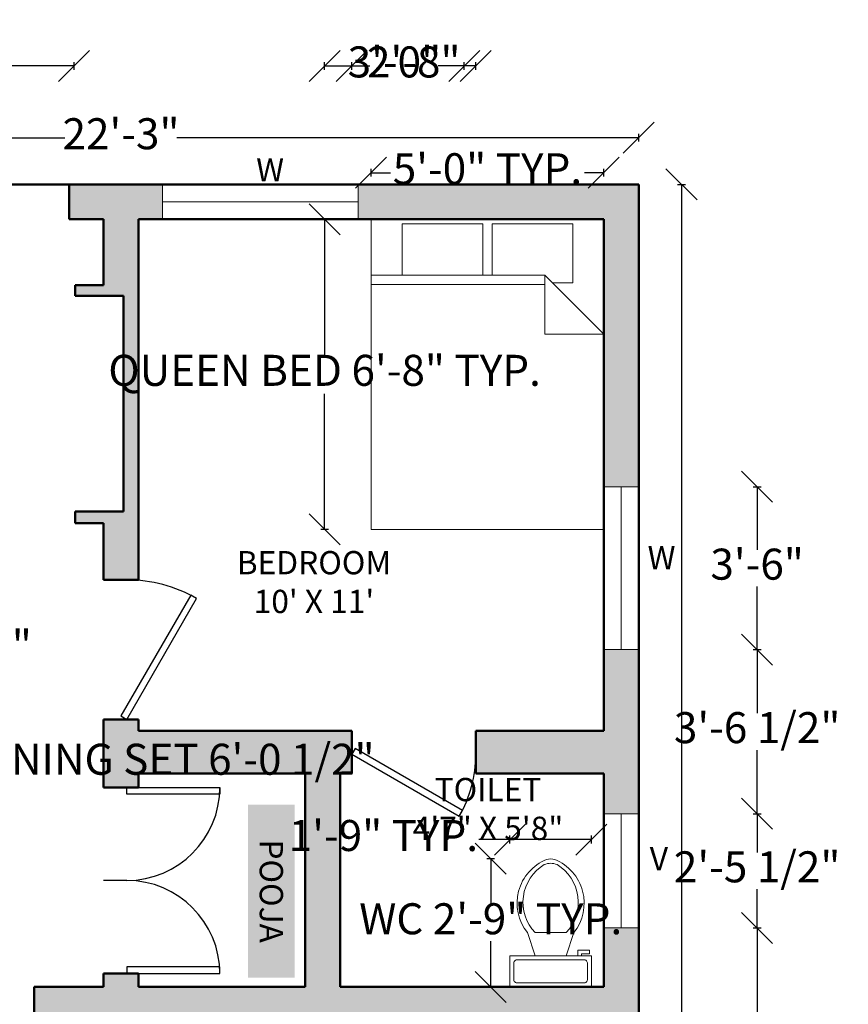
# Model space of a CAD drawing. Units: inches. Extents: x 3121 to 3511, y 1323 to 1998.
# Tile 10 of 10: x 3297 to 3511, y 1744 to 1998. Entities that reach past the tile are written whole.
import ezdxf

# ---------------------------------------------------------------- set-up
doc = ezdxf.new("R2010")
doc.units = ezdxf.units.IN
for name, color, linetype, lineweight in [('A-ANNO-DIMS', 2, 'Continuous', 18), ('A-ANNO-TEXT', 7, 'Continuous', 18), ('A-AREA-IDEN', 7, 'Continuous', 25), ('A-DOOR', 3, 'Continuous', 25), ('A-FLOR-FIXT', 9, 'Continuous', 18), ('A-FURN', 8, 'Continuous', 18), ('A-GLAZ', 4, 'Continuous', 18), ('A-WALL', 7, 'Continuous', 50), ('A-WALL-PATT', 3, 'Continuous', 13)]:
    doc.layers.add(name, color=color, linetype=linetype, lineweight=lineweight)
doc.styles.get("Standard").update_dxf_attribs({"font": 'arial.ttf'})
doc.dimstyles.new('ISO-25', dxfattribs={"dimtxt": 8, "dimasz": 8, "dimexe": 1, "dimexo": 1, "dimtad": 0, "dimtih": 1, "dimtoh": 1, "dimlunit": 3, "dimtxsty": 'Standard', "dimblk": 'OBLIQUE', "dimcen": 2.5, "dimclrt": 1, "dimadec": 0, "dimazin": 0, "dimtfac": 1, "dimtmove": 0, "dimatfit": 3, "dimfxl": 1, "dimfxlon": 1, "dimarcsym": 0})

# ---------------------------------------------------------------- blocks, each defined once
blk = doc.blocks.new('Bed - Queen')
for p, q in [((0, -80.00003), (0, 0)), ((0, 0), (59.99999, 0)), ((59.99999, 0), (59.99999, -80.00003)), ((7.99999, -1.2), (28.79998, -1.2)), ((7.99999, -14.4), (7.99999, -1.2)), ((28.79998, -1.2), (28.79998, -14.4)), ((31.19999, -1.2), (51.99999, -1.2)), ((31.19999, -14.4), (31.19999, -1.2)), ((51.99999, -1.2), (51.99999, -16.4)), ((0, -14.4), (44.8, -14.4)), ((59.99999, -29.6), (44.8, -14.4)), ((44.8, -14.4), (44.8, -29.6)), ((44.8, -16.8), (0, -16.8)), ((51.99999, -16.4), (46.79936, -16.4)), ((44.8, -29.6), (59.99999, -29.6)), ((59.99999, -80.00003), (0, -80.00003))]:
    blk.add_line(p, q)
blk = doc.blocks.new('Toilet - top')
for p, q in [((9.5, -6), (9.5, -2)), ((-10, -8.5), (-8, -8.5)), ((-10, -9.5), (-10, -8.5)), ((-7, -9.5), (-10, -9.5)), ((-8, -8.5), (-8, -8)), ((-7, -8), (-7, -9.5)), ((-4, -8), (-6, -14)), ((4, -8), (6, -14)), ((4, -14), (-4, -14))]:
    blk.add_line(p, q)
blk.add_lwpolyline([(10.5, -8), (10.5, 0), (-10.5, 0), (-10.5, -8)], close=True)
for points in [[(-9.5, -2), (-9.5, -6)], [(8.5, -1), (-8.5, -1)], [(-8.5, -7), (8.5, -7)]]:
    blk.add_lwpolyline(points)
for centre, radius, start, end in [((-8.62, -1.88), 0.884, 81.8699, 188.1301), ((8.62, -1.88), 0.884, 351.8699, 98.1301), ((-8.62, -6.12), 0.884, 171.8699, 278.1301), ((8.62, -6.12), 0.884, 261.8699, 8.1301), ((3.52, -21.58), 12.17, 141.4691, 247.9714), ((4.2, -21.82), 11.33, 136.3677, 238.9468), ((-3.52, -21.58), 12.17, 292.0284, 38.5307), ((-4.2, -21.82), 11.33, 301.053, 43.6321), ((0, -27.88), 4, 245.7318, 294.2682), ((0, -29), 4, 254.8605, 285.1395)]:
    blk.add_arc(centre, radius, start, end)
blk = doc.blocks.new('*U15')
for p, q in [((0, 0), (0, -6)), ((24, 0), (24, -6))]:
    blk.add_line(p, q)
blk.add_lwpolyline([(0, 0), (0, 24), (1.75, 24), (1.75, 0)], close=True)
blk.add_arc((0, 0), 24, 0, 90)
blk = doc.blocks.new('*U16')
for p, q in [((0, 0), (0, 6)), ((32, 0), (32, 6))]:
    blk.add_line(p, q)
blk.add_lwpolyline([(0, 0), (27.71, -16), (28.59, -14.48), (0.87, 1.52)], close=True)
blk.add_arc((0, 0), 32, 330, 0)
blk = doc.blocks.new('*U12')
for p, q in [((0, 0), (0, -6)), ((-36, 0), (-36, -6))]:
    blk.add_line(p, q)
blk.add_lwpolyline([(0, 0), (-31.18, 18), (-32.05, 16.48), (-0.88, -1.52)], close=True)
blk.add_arc((0, 0), 36, 150, 180)
blk = doc.blocks.new('*U14')
for p, q in [((-24, 0), (-24, -6)), ((0, 0), (0, -6))]:
    blk.add_line(p, q)
blk.add_lwpolyline([(0, 0), (0, 24), (-1.75, 24), (-1.75, 0)], close=True)
blk.add_arc((0, 0), 24, 90, 180)
blk = doc.blocks.new('_Oblique')
at = {"color": 0, "linetype": 'ByBlock', "lineweight": -2}
blk.add_line((-0.5, -0.5), (0.5, 0.5), dxfattribs=at)
blk = doc.blocks.new('*D17')
at = {"layer": 'A-ANNO-DIMS', "color": 0, "lineweight": -2, "transparency": 16777216}
for p, q in [((3189.92, 1966.81), (3189.92, 1968.81)), ((3456.92, 1966.81), (3456.92, 1968.81)), ((3189.92, 1967.81), (3308.98, 1967.81)), ((3456.92, 1967.81), (3337.85, 1967.81))]:
    blk.add_line(p, q, dxfattribs=at)
at = {"layer": 'Defpoints', "color": 0, "transparency": 16777216}
for p in [(3456.92, 1967.81), (3189.92, 1955.78), (3456.92, 1955.78)]:
    blk.add_point(p, dxfattribs=at)
at = {"layer": 'A-ANNO-DIMS', "color": 0, "lineweight": -2, "transparency": 16777216, "xscale": 8, "yscale": 8, "zscale": 8, "rotation": 180}
blk.add_blockref('_Oblique', (3189.92, 1967.81), dxfattribs=at)
at = {"layer": 'A-ANNO-DIMS', "color": 0, "lineweight": -2, "transparency": 16777216, "xscale": 8, "yscale": 8, "zscale": 8}
blk.add_blockref('_Oblique', (3456.92, 1967.81), dxfattribs=at)
at = {"layer": 'A-ANNO-DIMS', "color": 0, "transparency": 16777216, "insert": (3323.42, 1967.81), "char_height": 8, "attachment_point": 5}
blk.add_mtext('22\'-3"', dxfattribs=at)
blk = doc.blocks.new('*D18')
at = {"layer": 'A-ANNO-DIMS', "color": 0, "lineweight": -2, "transparency": 16777216}
for p, q in [((3466.96, 1955.78), (3468.96, 1955.78)), ((3467.96, 1955.78), (3467.96, 1690.48)), ((3467.96, 1415.78), (3467.96, 1681.09)), ((3466.96, 1415.78), (3468.96, 1415.78))]:
    blk.add_line(p, q, dxfattribs=at)
at = {"layer": 'Defpoints', "color": 0, "transparency": 16777216}
for p in [(3456.92, 1955.78), (3456.92, 1415.78), (3467.96, 1415.78)]:
    blk.add_point(p, dxfattribs=at)
at = {"layer": 'A-ANNO-DIMS', "color": 0, "lineweight": -2, "transparency": 16777216, "xscale": 8, "yscale": 8, "zscale": 8}
for p, rotation in [((3467.96, 1955.78), 90), ((3467.96, 1415.78), 270)]:
    blk.add_blockref('_Oblique', p, dxfattribs=dict(at, rotation=rotation))
at = {"layer": 'A-ANNO-DIMS', "color": 0, "transparency": 16777216, "insert": (3467.96, 1685.78), "char_height": 8, "attachment_point": 5}
blk.add_mtext("45'", dxfattribs=at)
blk = doc.blocks.new('*D19')
at = {"layer": 'A-ANNO-DIMS', "color": 0, "lineweight": -2, "transparency": 16777216}
for p, q in [((3376.92, 1946.78), (3374.92, 1946.78)), ((3375.92, 1946.78), (3375.92, 1911.79)), ((3375.92, 1866.78), (3375.92, 1901.78)), ((3376.92, 1866.78), (3374.92, 1866.78))]:
    blk.add_line(p, q, dxfattribs=at)
at = {"layer": 'Defpoints', "color": 0, "transparency": 16777216}
for p in [(3375.92, 1946.78), (3387.92, 1946.78), (3387.92, 1866.78)]:
    blk.add_point(p, dxfattribs=at)
at = {"layer": 'A-ANNO-DIMS', "color": 0, "lineweight": -2, "transparency": 16777216, "xscale": 8, "yscale": 8, "zscale": 8}
for p, rotation in [((3375.92, 1946.78), 90), ((3375.92, 1866.78), 270)]:
    blk.add_blockref('_Oblique', p, dxfattribs=dict(at, rotation=rotation))
at = {"layer": 'A-ANNO-DIMS', "color": 1, "transparency": 16777216, "insert": (3375.92, 1906.78), "char_height": 8, "attachment_point": 5}
blk.add_mtext('QUEEN BED 6\'-8" TYP.', dxfattribs=at)
blk = doc.blocks.new('*D20')
at = {"layer": 'A-ANNO-DIMS', "color": 0, "lineweight": -2, "transparency": 16777216}
for p, q in [((3387.92, 1957.78), (3387.92, 1959.78)), ((3387.92, 1958.78), (3392.91, 1958.78)), ((3447.92, 1958.78), (3442.93, 1958.78)), ((3447.92, 1957.78), (3447.92, 1959.78))]:
    blk.add_line(p, q, dxfattribs=at)
at = {"layer": 'Defpoints', "color": 0, "transparency": 16777216}
for p in [(3447.92, 1958.78), (3387.92, 1946.78), (3447.92, 1946.78)]:
    blk.add_point(p, dxfattribs=at)
at = {"layer": 'A-ANNO-DIMS', "color": 0, "lineweight": -2, "transparency": 16777216, "xscale": 8, "yscale": 8, "zscale": 8, "rotation": 180}
blk.add_blockref('_Oblique', (3387.92, 1958.78), dxfattribs=at)
at = {"layer": 'A-ANNO-DIMS', "color": 0, "lineweight": -2, "transparency": 16777216, "xscale": 8, "yscale": 8, "zscale": 8}
blk.add_blockref('_Oblique', (3447.92, 1958.78), dxfattribs=at)
at = {"layer": 'A-ANNO-DIMS', "color": 1, "transparency": 16777216, "insert": (3417.92, 1958.78), "char_height": 8, "attachment_point": 5}
blk.add_mtext('5\'-0" TYP.', dxfattribs=at)
blk = doc.blocks.new('*D23')
at = {"layer": 'A-ANNO-DIMS', "color": 0, "lineweight": -2, "transparency": 16777216}
for p, q in [((3419.76, 1781.83), (3417.76, 1781.83)), ((3418.76, 1781.83), (3418.76, 1770.07)), ((3418.76, 1748.78), (3418.76, 1760.55)), ((3419.76, 1748.78), (3417.76, 1748.78))]:
    blk.add_line(p, q, dxfattribs=at)
at = {"layer": 'Defpoints', "color": 0, "transparency": 16777216}
for p in [(3423.72, 1781.83), (3418.76, 1748.78), (3423.72, 1748.78)]:
    blk.add_point(p, dxfattribs=at)
at = {"layer": 'A-ANNO-DIMS', "color": 0, "lineweight": -2, "transparency": 16777216, "xscale": 8, "yscale": 8, "zscale": 8}
for p, rotation in [((3418.76, 1781.83), 90), ((3418.76, 1748.78), 270)]:
    blk.add_blockref('_Oblique', p, dxfattribs=dict(at, rotation=rotation))
at = {"layer": 'A-ANNO-DIMS', "color": 1, "transparency": 16777216, "insert": (3418.76, 1765.31), "char_height": 8, "attachment_point": 5}
blk.add_mtext('WC 2\'-9" TYP.', dxfattribs=at)
blk = doc.blocks.new('*D24')
at = {"layer": 'A-ANNO-DIMS', "color": 0, "lineweight": -2, "transparency": 16777216}
for p, q in [((3423.72, 1786.79), (3415.72, 1786.79)), ((3423.72, 1785.79), (3423.72, 1787.79)), ((3444.72, 1786.79), (3423.72, 1786.79)), ((3444.72, 1785.79), (3444.72, 1787.79))]:
    blk.add_line(p, q, dxfattribs=at)
at = {"layer": 'Defpoints', "color": 0, "transparency": 16777216}
for p in [(3423.72, 1786.79), (3423.72, 1781.83), (3444.72, 1781.83)]:
    blk.add_point(p, dxfattribs=at)
at = {"layer": 'A-ANNO-DIMS', "color": 0, "lineweight": -2, "transparency": 16777216, "xscale": 8, "yscale": 8, "zscale": 8, "rotation": 180}
blk.add_blockref('_Oblique', (3423.72, 1786.79), dxfattribs=at)
at = {"layer": 'A-ANNO-DIMS', "color": 0, "lineweight": -2, "transparency": 16777216, "xscale": 8, "yscale": 8, "zscale": 8}
blk.add_blockref('_Oblique', (3444.72, 1786.79), dxfattribs=at)
at = {"layer": 'A-ANNO-DIMS', "color": 1, "transparency": 16777216, "insert": (3391.09, 1786.79), "char_height": 8, "attachment_point": 5}
blk.add_mtext('1\'-9" TYP.', dxfattribs=at)
blk = doc.blocks.new('*D27')
at = {"layer": 'A-ANNO-DIMS', "color": 0, "lineweight": -2, "transparency": 16777216}
for p, q in [((3202.09, 1805.46), (3202.09, 1807.46)), ((3202.09, 1806.46), (3274.67, 1806.46)), ((3274.67, 1805.46), (3274.67, 1807.46)), ((3274.67, 1806.46), (3282.67, 1806.46))]:
    blk.add_line(p, q, dxfattribs=at)
at = {"layer": 'Defpoints', "color": 0, "transparency": 16777216}
for p in [(3274.67, 1806.46), (3202.09, 1795.57), (3274.67, 1795.57)]:
    blk.add_point(p, dxfattribs=at)
at = {"layer": 'A-ANNO-DIMS', "color": 0, "lineweight": -2, "transparency": 16777216, "xscale": 8, "yscale": 8, "zscale": 8, "rotation": 180}
blk.add_blockref('_Oblique', (3202.09, 1806.46), dxfattribs=at)
at = {"layer": 'A-ANNO-DIMS', "color": 0, "lineweight": -2, "transparency": 16777216, "xscale": 8, "yscale": 8, "zscale": 8}
blk.add_blockref('_Oblique', (3274.67, 1806.46), dxfattribs=at)
at = {"layer": 'A-ANNO-DIMS', "color": 1, "transparency": 16777216, "insert": (3336.58, 1806.46), "char_height": 8, "attachment_point": 5}
blk.add_mtext('DINING SET 6\'-0 1/2"', dxfattribs=at)
blk = doc.blocks.new('*D48')
at = {"layer": 'A-ANNO-DIMS', "color": 0, "lineweight": -2, "transparency": 16777216}
for p, q in [((3486.47, 1763.99), (3488.47, 1763.99)), ((3487.47, 1763.99), (3487.47, 1682.6)), ((3487.47, 1591.7), (3487.47, 1673.08)), ((3486.47, 1591.7), (3488.47, 1591.7))]:
    blk.add_line(p, q, dxfattribs=at)
at = {"layer": 'Defpoints', "color": 0, "transparency": 16777216}
for p in [(3456.92, 1763.99), (3487.47, 1763.99), (3456.92, 1591.7)]:
    blk.add_point(p, dxfattribs=at)
at = {"layer": 'A-ANNO-DIMS', "color": 0, "lineweight": -2, "transparency": 16777216, "xscale": 8, "yscale": 8, "zscale": 8}
for p, rotation in [((3487.47, 1763.99), 90), ((3487.47, 1591.7), 270)]:
    blk.add_blockref('_Oblique', p, dxfattribs=dict(at, rotation=rotation))
at = {"layer": 'A-ANNO-DIMS', "color": 1, "transparency": 16777216, "insert": (3487.47, 1677.84), "char_height": 8, "attachment_point": 5}
blk.add_mtext('14\'-4 1/2"', dxfattribs=at)
blk = doc.blocks.new('*D49')
at = {"layer": 'A-ANNO-DIMS', "color": 0, "lineweight": -2, "transparency": 16777216}
for p, q in [((3486.47, 1793.44), (3488.47, 1793.44)), ((3487.47, 1793.44), (3487.47, 1783.48)), ((3487.47, 1763.99), (3487.47, 1773.95)), ((3486.47, 1763.99), (3488.47, 1763.99))]:
    blk.add_line(p, q, dxfattribs=at)
at = {"layer": 'Defpoints', "color": 0, "transparency": 16777216}
for p in [(3456.92, 1793.44), (3487.47, 1793.44), (3456.92, 1763.99)]:
    blk.add_point(p, dxfattribs=at)
at = {"layer": 'A-ANNO-DIMS', "color": 0, "lineweight": -2, "transparency": 16777216, "xscale": 8, "yscale": 8, "zscale": 8}
for p, rotation in [((3487.47, 1793.44), 90), ((3487.47, 1763.99), 270)]:
    blk.add_blockref('_Oblique', p, dxfattribs=dict(at, rotation=rotation))
at = {"layer": 'A-ANNO-DIMS', "color": 1, "transparency": 16777216, "insert": (3487.47, 1778.71), "char_height": 8, "attachment_point": 5}
blk.add_mtext('2\'-5 1/2"', dxfattribs=at)
blk = doc.blocks.new('*D50')
at = {"layer": 'A-ANNO-DIMS', "color": 0, "lineweight": -2, "transparency": 16777216}
for p, q in [((3486.47, 1835.78), (3488.47, 1835.78)), ((3487.47, 1835.78), (3487.47, 1819.38)), ((3487.47, 1793.44), (3487.47, 1809.85)), ((3486.47, 1793.44), (3488.47, 1793.44))]:
    blk.add_line(p, q, dxfattribs=at)
at = {"layer": 'Defpoints', "color": 0, "transparency": 16777216}
for p in [(3456.92, 1835.78), (3487.47, 1835.78), (3456.92, 1793.44)]:
    blk.add_point(p, dxfattribs=at)
at = {"layer": 'A-ANNO-DIMS', "color": 0, "lineweight": -2, "transparency": 16777216, "xscale": 8, "yscale": 8, "zscale": 8}
for p, rotation in [((3487.47, 1835.78), 90), ((3487.47, 1793.44), 270)]:
    blk.add_blockref('_Oblique', p, dxfattribs=dict(at, rotation=rotation))
at = {"layer": 'A-ANNO-DIMS', "color": 1, "transparency": 16777216, "insert": (3487.47, 1814.61), "char_height": 8, "attachment_point": 5}
blk.add_mtext('3\'-6 1/2"', dxfattribs=at)
blk = doc.blocks.new('*D51')
at = {"layer": 'A-ANNO-DIMS', "color": 0, "lineweight": -2, "transparency": 16777216}
for p, q in [((3486.47, 1877.78), (3488.47, 1877.78)), ((3487.47, 1877.78), (3487.47, 1861.49)), ((3487.47, 1835.78), (3487.47, 1852.07)), ((3486.47, 1835.78), (3488.47, 1835.78))]:
    blk.add_line(p, q, dxfattribs=at)
at = {"layer": 'Defpoints', "color": 0, "transparency": 16777216}
for p in [(3456.92, 1877.78), (3487.47, 1877.78), (3456.92, 1835.78)]:
    blk.add_point(p, dxfattribs=at)
at = {"layer": 'A-ANNO-DIMS', "color": 0, "lineweight": -2, "transparency": 16777216, "xscale": 8, "yscale": 8, "zscale": 8}
for p, rotation in [((3487.47, 1877.78), 90), ((3487.47, 1835.78), 270)]:
    blk.add_blockref('_Oblique', p, dxfattribs=dict(at, rotation=rotation))
at = {"layer": 'A-ANNO-DIMS', "color": 1, "transparency": 16777216, "insert": (3487.47, 1856.78), "char_height": 8, "attachment_point": 5}
blk.add_mtext('3\'-6"', dxfattribs=at)
blk = doc.blocks.new('*D53')
at = {"layer": 'A-ANNO-DIMS', "color": 0, "lineweight": -2, "transparency": 16777216}
for p, q in [((3274.02, 1336.37), (3274.02, 1334.37)), ((3310.02, 1336.37), (3310.02, 1334.37)), ((3274.02, 1335.37), (3280.77, 1335.37)), ((3310.02, 1335.37), (3303.28, 1335.37))]:
    blk.add_line(p, q, dxfattribs=at)
at = {"layer": 'Defpoints', "color": 0, "transparency": 16777216}
for p in [(3274.02, 1946.78), (3310.02, 1946.78), (3310.02, 1335.37)]:
    blk.add_point(p, dxfattribs=at)
at = {"layer": 'A-ANNO-DIMS', "color": 0, "lineweight": -2, "transparency": 16777216, "xscale": 8, "yscale": 8, "zscale": 8, "rotation": 180}
blk.add_blockref('_Oblique', (3274.02, 1335.37), dxfattribs=at)
at = {"layer": 'A-ANNO-DIMS', "color": 0, "lineweight": -2, "transparency": 16777216, "xscale": 8, "yscale": 8, "zscale": 8}
blk.add_blockref('_Oblique', (3310.02, 1335.37), dxfattribs=at)
at = {"layer": 'A-ANNO-DIMS', "color": 1, "transparency": 16777216, "insert": (3292.02, 1335.37), "char_height": 8, "attachment_point": 5}
blk.add_mtext('3\'-0"', dxfattribs=at)
blk = doc.blocks.new('*D54')
at = {"layer": 'A-ANNO-DIMS', "color": 0, "lineweight": -2, "transparency": 16777216}
for p, q in [((3310.02, 1336.37), (3310.02, 1334.37)), ((3334.16, 1336.37), (3334.16, 1334.37)), ((3310.02, 1335.37), (3310.76, 1335.37)), ((3334.16, 1335.37), (3333.42, 1335.37))]:
    blk.add_line(p, q, dxfattribs=at)
at = {"layer": 'Defpoints', "color": 0, "transparency": 16777216}
for p in [(3310.02, 1946.78), (3334.16, 1946.78), (3334.16, 1335.37)]:
    blk.add_point(p, dxfattribs=at)
at = {"layer": 'A-ANNO-DIMS', "color": 0, "lineweight": -2, "transparency": 16777216, "xscale": 8, "yscale": 8, "zscale": 8, "rotation": 180}
blk.add_blockref('_Oblique', (3310.02, 1335.37), dxfattribs=at)
at = {"layer": 'A-ANNO-DIMS', "color": 0, "lineweight": -2, "transparency": 16777216, "xscale": 8, "yscale": 8, "zscale": 8}
blk.add_blockref('_Oblique', (3334.16, 1335.37), dxfattribs=at)
at = {"layer": 'A-ANNO-DIMS', "color": 1, "transparency": 16777216, "insert": (3322.09, 1335.37), "char_height": 8, "attachment_point": 5}
blk.add_mtext('2\'-0"', dxfattribs=at)
blk = doc.blocks.new('*D55')
at = {"layer": 'A-ANNO-DIMS', "color": 0, "lineweight": -2, "transparency": 16777216}
for p, q in [((3334.16, 1336.37), (3334.16, 1334.37)), ((3384.56, 1336.37), (3384.56, 1334.37)), ((3334.16, 1335.37), (3338.62, 1335.37)), ((3384.56, 1335.37), (3380.1, 1335.37))]:
    blk.add_line(p, q, dxfattribs=at)
at = {"layer": 'Defpoints', "color": 0, "transparency": 16777216}
for p in [(3334.16, 1946.78), (3384.56, 1946.78), (3384.56, 1335.37)]:
    blk.add_point(p, dxfattribs=at)
at = {"layer": 'A-ANNO-DIMS', "color": 0, "lineweight": -2, "transparency": 16777216, "xscale": 8, "yscale": 8, "zscale": 8, "rotation": 180}
blk.add_blockref('_Oblique', (3334.16, 1335.37), dxfattribs=at)
at = {"layer": 'A-ANNO-DIMS', "color": 0, "lineweight": -2, "transparency": 16777216, "xscale": 8, "yscale": 8, "zscale": 8}
blk.add_blockref('_Oblique', (3384.56, 1335.37), dxfattribs=at)
at = {"layer": 'A-ANNO-DIMS', "color": 1, "transparency": 16777216, "insert": (3359.36, 1335.37), "char_height": 8, "attachment_point": 5}
blk.add_mtext('4\'-2 1/2"', dxfattribs=at)
blk = doc.blocks.new('*D58')
at = {"layer": 'A-ANNO-DIMS', "color": 0, "lineweight": -2, "transparency": 16777216}
for p, q in [((3209.89, 1985.33), (3209.89, 1987.33)), ((3209.89, 1986.33), (3240.03, 1986.33)), ((3311.33, 1986.33), (3281.19, 1986.33)), ((3311.33, 1985.33), (3311.33, 1987.33))]:
    blk.add_line(p, q, dxfattribs=at)
at = {"layer": 'Defpoints', "color": 0, "transparency": 16777216}
for p in [(3311.33, 1986.33), (3209.89, 1424.78), (3311.33, 1424.78)]:
    blk.add_point(p, dxfattribs=at)
at = {"layer": 'A-ANNO-DIMS', "color": 0, "lineweight": -2, "transparency": 16777216, "xscale": 8, "yscale": 8, "zscale": 8, "rotation": 180}
blk.add_blockref('_Oblique', (3209.89, 1986.33), dxfattribs=at)
at = {"layer": 'A-ANNO-DIMS', "color": 0, "lineweight": -2, "transparency": 16777216, "xscale": 8, "yscale": 8, "zscale": 8}
blk.add_blockref('_Oblique', (3311.33, 1986.33), dxfattribs=at)
at = {"layer": 'A-ANNO-DIMS', "color": 1, "transparency": 16777216, "insert": (3260.61, 1986.33), "char_height": 8, "attachment_point": 5}
blk.add_mtext('8\'-5 1/2"', dxfattribs=at)
blk = doc.blocks.new('*D59')
at = {"layer": 'A-ANNO-DIMS', "color": 0, "lineweight": -2, "transparency": 16777216}
for p, q in [((3318.92, 1336.37), (3318.92, 1334.37)), ((3370.92, 1336.37), (3370.92, 1334.37)), ((3318.92, 1335.37), (3333.5, 1335.37)), ((3370.92, 1335.37), (3356.34, 1335.37))]:
    blk.add_line(p, q, dxfattribs=at)
at = {"layer": 'Defpoints', "color": 0, "transparency": 16777216}
for p in [(3318.92, 1752.23), (3370.92, 1748.78), (3370.92, 1335.37)]:
    blk.add_point(p, dxfattribs=at)
at = {"layer": 'A-ANNO-DIMS', "color": 0, "lineweight": -2, "transparency": 16777216, "xscale": 8, "yscale": 8, "zscale": 8, "rotation": 180}
blk.add_blockref('_Oblique', (3318.92, 1335.37), dxfattribs=at)
at = {"layer": 'A-ANNO-DIMS', "color": 0, "lineweight": -2, "transparency": 16777216, "xscale": 8, "yscale": 8, "zscale": 8}
blk.add_blockref('_Oblique', (3370.92, 1335.37), dxfattribs=at)
at = {"layer": 'A-ANNO-DIMS', "color": 1, "transparency": 16777216, "insert": (3344.92, 1335.37), "char_height": 8, "attachment_point": 5}
blk.add_mtext('4\'-4"', dxfattribs=at)
blk = doc.blocks.new('*D60')
at = {"layer": 'A-ANNO-DIMS', "color": 0, "lineweight": -2, "transparency": 16777216}
for p, q in [((3160.368016, 1803.784138), (3158.368016, 1803.784138)), ((3159.368016, 1803.784138), (3159.368016, 1780.909138)), ((3159.368016, 1748.784138), (3159.368016, 1771.659138)), ((3160.368016, 1748.784138), (3158.368016, 1748.784138))]:
    blk.add_line(p, q, dxfattribs=at)
at = {"layer": 'Defpoints', "color": 0, "transparency": 16777216}
for p in [(3159.368016, 1803.784138), (3370.918016, 1803.784138), (3370.918016, 1748.784138)]:
    blk.add_point(p, dxfattribs=at)
at = {"layer": 'A-ANNO-DIMS', "color": 0, "lineweight": -2, "transparency": 16777216, "xscale": 8, "yscale": 8, "zscale": 8}
for p, rotation in [((3159.368016, 1803.784138), 90), ((3159.368016, 1748.784138), 270)]:
    blk.add_blockref('_Oblique', p, dxfattribs=dict(at, rotation=rotation))
at = {"layer": 'A-ANNO-DIMS', "color": 1, "transparency": 16777216, "insert": (3159.368016, 1776.284138), "char_height": 8, "attachment_point": 5}
blk.add_mtext('4\'-7"', dxfattribs=at)
blk = doc.blocks.new('*D61')
at = {"layer": 'A-ANNO-DIMS', "color": 0, "lineweight": -2, "transparency": 16777216}
for p, q in [((3382.92, 1985.33), (3382.92, 1987.33)), ((3382.92, 1986.33), (3387.59, 1986.33)), ((3414.92, 1986.33), (3410.24, 1986.33)), ((3414.92, 1985.33), (3414.92, 1987.33))]:
    blk.add_line(p, q, dxfattribs=at)
at = {"layer": 'Defpoints', "color": 0, "transparency": 16777216}
for p in [(3414.92, 1986.33), (3382.92, 1814.78), (3414.92, 1814.78)]:
    blk.add_point(p, dxfattribs=at)
at = {"layer": 'A-ANNO-DIMS', "color": 0, "lineweight": -2, "transparency": 16777216, "xscale": 8, "yscale": 8, "zscale": 8, "rotation": 180}
blk.add_blockref('_Oblique', (3382.92, 1986.33), dxfattribs=at)
at = {"layer": 'A-ANNO-DIMS', "color": 0, "lineweight": -2, "transparency": 16777216, "xscale": 8, "yscale": 8, "zscale": 8}
blk.add_blockref('_Oblique', (3414.92, 1986.33), dxfattribs=at)
at = {"layer": 'A-ANNO-DIMS', "color": 1, "transparency": 16777216, "insert": (3398.92, 1986.33), "char_height": 8, "attachment_point": 5}
blk.add_mtext('2\'-8"', dxfattribs=at)
blk = doc.blocks.new('*D62')
at = {"layer": 'A-ANNO-DIMS', "color": 0, "lineweight": -2, "transparency": 16777216}
for p, q in [((3160.37, 1800.22), (3158.37, 1800.22)), ((3159.37, 1800.22), (3159.37, 1780.93)), ((3159.37, 1752.23), (3159.37, 1771.52)), ((3160.37, 1752.23), (3158.37, 1752.23))]:
    blk.add_line(p, q, dxfattribs=at)
at = {"layer": 'Defpoints', "color": 0, "transparency": 16777216}
for p in [(3159.37, 1800.22), (3318.92, 1800.22), (3318.92, 1752.23)]:
    blk.add_point(p, dxfattribs=at)
at = {"layer": 'A-ANNO-DIMS', "color": 0, "lineweight": -2, "transparency": 16777216, "xscale": 8, "yscale": 8, "zscale": 8}
for p, rotation in [((3159.37, 1800.22), 90), ((3159.37, 1752.23), 270)]:
    blk.add_blockref('_Oblique', p, dxfattribs=dict(at, rotation=rotation))
at = {"layer": 'A-ANNO-DIMS', "color": 1, "transparency": 16777216, "insert": (3159.37, 1776.22), "char_height": 8, "attachment_point": 5}
blk.add_mtext('4\'-0"', dxfattribs=at)
blk = doc.blocks.new('*D63')
at = {"layer": 'A-ANNO-DIMS', "color": 0, "lineweight": -2, "transparency": 16777216}
for p, q in [((3370.92, 1336.37), (3370.92, 1334.37)), ((3379.92, 1336.37), (3379.92, 1334.37)), ((3370.92, 1335.37), (3379.92, 1335.37)), ((3379.92, 1335.37), (3387.92, 1335.37))]:
    blk.add_line(p, q, dxfattribs=at)
at = {"layer": 'Defpoints', "color": 0, "transparency": 16777216}
for p in [(3370.92, 1748.78), (3379.92, 1748.78), (3379.92, 1335.37)]:
    blk.add_point(p, dxfattribs=at)
at = {"layer": 'A-ANNO-DIMS', "color": 0, "lineweight": -2, "transparency": 16777216, "xscale": 8, "yscale": 8, "zscale": 8, "rotation": 180}
blk.add_blockref('_Oblique', (3370.92, 1335.37), dxfattribs=at)
at = {"layer": 'A-ANNO-DIMS', "color": 0, "lineweight": -2, "transparency": 16777216, "xscale": 8, "yscale": 8, "zscale": 8}
blk.add_blockref('_Oblique', (3379.92, 1335.37), dxfattribs=at)
at = {"layer": 'A-ANNO-DIMS', "color": 1, "transparency": 16777216, "insert": (3399.18, 1335.37), "char_height": 8, "attachment_point": 5}
blk.add_mtext('0\'-9"', dxfattribs=at)
blk = doc.blocks.new('*D74')
at = {"layer": 'A-ANNO-DIMS', "color": 0, "lineweight": -2, "transparency": 16777216}
for p, q in [((3375.92, 1985.33), (3375.92, 1987.33)), ((3375.92, 1986.33), (3382.66, 1986.33)), ((3411.92, 1986.33), (3405.17, 1986.33)), ((3411.92, 1985.33), (3411.92, 1987.33))]:
    blk.add_line(p, q, dxfattribs=at)
at = {"layer": 'Defpoints', "color": 0, "transparency": 16777216}
for p in [(3411.92, 1986.33), (3375.92, 1674.28), (3411.92, 1674.28)]:
    blk.add_point(p, dxfattribs=at)
at = {"layer": 'A-ANNO-DIMS', "color": 0, "lineweight": -2, "transparency": 16777216, "xscale": 8, "yscale": 8, "zscale": 8, "rotation": 180}
blk.add_blockref('_Oblique', (3375.92, 1986.33), dxfattribs=at)
at = {"layer": 'A-ANNO-DIMS', "color": 0, "lineweight": -2, "transparency": 16777216, "xscale": 8, "yscale": 8, "zscale": 8}
blk.add_blockref('_Oblique', (3411.92, 1986.33), dxfattribs=at)
at = {"layer": 'A-ANNO-DIMS', "color": 1, "transparency": 16777216, "insert": (3393.92, 1986.33), "char_height": 8, "attachment_point": 5}
blk.add_mtext('3\'-0"', dxfattribs=at)
blk = doc.blocks.new('*D78')
at = {"layer": 'A-ANNO-DIMS', "color": 0, "lineweight": -2, "transparency": 16777216}
for p, q in [((3289.37, 1853.78), (3287.37, 1853.78)), ((3288.37, 1853.78), (3288.37, 1840.5)), ((3288.37, 1817.78), (3288.37, 1831.07)), ((3289.37, 1817.78), (3287.37, 1817.78))]:
    blk.add_line(p, q, dxfattribs=at)
at = {"layer": 'Defpoints', "color": 0, "transparency": 16777216}
for p in [(3288.37, 1853.78), (3318.92, 1853.78), (3318.92, 1817.78)]:
    blk.add_point(p, dxfattribs=at)
at = {"layer": 'A-ANNO-DIMS', "color": 0, "lineweight": -2, "transparency": 16777216, "xscale": 8, "yscale": 8, "zscale": 8}
for p, rotation in [((3288.37, 1853.78), 90), ((3288.37, 1817.78), 270)]:
    blk.add_blockref('_Oblique', p, dxfattribs=dict(at, rotation=rotation))
at = {"layer": 'A-ANNO-DIMS', "color": 1, "transparency": 16777216, "insert": (3288.37, 1835.78), "char_height": 8, "attachment_point": 5}
blk.add_mtext('3\'-0"', dxfattribs=at)

msp = doc.modelspace()

# ---------------------------------------------------------------- hatches: boundary and pattern name
at = {"layer": 'A-WALL-PATT'}
h = msp.add_hatch(color=256, dxfattribs=at)
h.dxf.hatch_style = 1
h.paths.add_polyline_path([(3274.023, 1955.784), (3189.918, 1955.784), (3189.918, 1910.219), (3198.918, 1910.219), (3198.918, 1946.784), (3259.023, 1946.784), (3259.023, 1921.61), (3261.023, 1921.61), (3261.023, 1946.784), (3274.023, 1946.784)])
h.paths.add_polyline_path([(3327.918, 1946.784), (3334.156, 1946.784), (3334.156, 1955.784), (3310.023, 1955.784), (3310.023, 1946.784), (3318.918, 1946.784), (3318.918, 1929.796), (3311.644, 1929.796), (3311.644, 1927.007), (3324.033, 1927.007), (3324.033, 1871.381), (3311.644, 1871.381), (3311.644, 1868.381), (3318.918, 1868.381), (3318.918, 1853.784), (3327.918, 1853.784)])
h.paths.add_polyline_path([(3456.918, 1955.784), (3384.562, 1955.784), (3384.562, 1946.784), (3447.918, 1946.784), (3447.918, 1877.779), (3456.918, 1877.779)])
h.paths.add_polyline_path([(3456.918, 1835.782), (3447.918, 1835.782), (3447.918, 1814.784), (3414.918, 1814.784), (3414.918, 1803.784), (3447.918, 1803.784), (3447.918, 1793.443), (3456.918, 1793.443)])
h.paths.add_polyline_path([(3456.918, 1558.434), (3447.918, 1558.434), (3447.918, 1547.784), (3375.918, 1547.784), (3375.918, 1598.784), (3378.918, 1598.784), (3378.918, 1602.284), (3375.918, 1602.284), (3375.918, 1674.284), (3369.918, 1674.284), (3369.918, 1547.784), (3364.418, 1547.784), (3364.418, 1538.784), (3447.918, 1538.784), (3447.918, 1512.628), (3456.918, 1512.628)])
h.paths.add_polyline_path([(3456.918, 1460.558), (3447.918, 1460.558), (3447.918, 1424.784), (3412.543, 1424.784), (3412.543, 1415.784), (3456.918, 1415.784)])
h.paths.add_polyline_path([(3358.149, 1424.784), (3322.918, 1424.784), (3322.918, 1538.784), (3328.418, 1538.784), (3328.418, 1547.784), (3308.208, 1547.784), (3308.208, 1538.784), (3318.918, 1538.784), (3318.918, 1424.784), (3311.328, 1424.784), (3311.328, 1415.784), (3358.149, 1415.784)])
h.paths.add_polyline_path([(3207.562, 1547.784), (3198.918, 1547.784), (3198.918, 1607.327), (3189.918, 1607.327), (3189.918, 1513.073), (3198.918, 1513.073), (3198.918, 1538.784), (3207.562, 1538.784)])
h.paths.add_polyline_path([(3198.918, 1461.548), (3189.918, 1461.548), (3189.918, 1415.784), (3209.892, 1415.784), (3209.892, 1424.784), (3198.918, 1424.784)])
h.paths.add_polyline_path([(3272.208, 1547.784), (3238.766, 1547.784), (3238.766, 1538.784), (3272.208, 1538.784)])
h.paths.add_polyline_path([(3261.023, 1748.784), (3198.918, 1748.784), (3198.918, 1768.387), (3189.918, 1768.387), (3189.918, 1692.279), (3198.918, 1692.279), (3198.918, 1739.784), (3261.023, 1739.784)])
h.paths.add_polyline_path([(3198.918, 1856.171), (3189.918, 1856.171), (3189.918, 1808.331), (3198.918, 1808.331), (3198.918, 1821.074), (3261.023, 1821.074), (3261.023, 1862.309), (3259.023, 1862.309), (3259.023, 1825.074), (3198.918, 1825.074)])
h = msp.add_hatch(color=256, dxfattribs=at)
h.dxf.hatch_style = 1
h.paths.add_polyline_path([(3382.918, 1814.784), (3327.918, 1814.784), (3327.918, 1817.784), (3318.918, 1817.784), (3318.918, 1800.224), (3324.918, 1800.224), (3327.918, 1800.224), (3327.918, 1803.784), (3370.918, 1803.784), (3370.918, 1748.784), (3327.918, 1748.784), (3327.918, 1752.226), (3324.918, 1752.226), (3318.918, 1752.226), (3318.918, 1748.784), (3301.026, 1748.784), (3301.026, 1739.784), (3447.918, 1739.784), (3447.918, 1602.284), (3418.918, 1602.284), (3418.918, 1598.784), (3447.918, 1598.784), (3447.918, 1591.697), (3456.918, 1591.697), (3456.918, 1763.985), (3447.918, 1763.985), (3447.918, 1748.784), (3379.918, 1748.784), (3379.918, 1803.784), (3382.918, 1803.784)])
h.paths.add_polyline_path([(3418.918, 1602.284), (3408.918, 1602.284), (3408.918, 1598.784), (3418.918, 1598.784)], flags=17)

# ---------------------------------------------------------------- linework, layer by layer
at = {"layer": 'A-GLAZ'}
for p, q in [((3334.156, 1946.784), (3334.156, 1955.784)), ((3384.562, 1955.784), (3384.562, 1946.784)), ((3334.156, 1951.284), (3384.562, 1951.284)), ((3447.918, 1877.779), (3456.918, 1877.779)), ((3452.418, 1877.779), (3452.418, 1835.782)), ((3447.918, 1835.782), (3456.918, 1835.782)), ((3447.918, 1793.443), (3456.918, 1793.443)), ((3452.418, 1763.985), (3452.418, 1793.443)), ((3447.918, 1763.985), (3456.918, 1763.985))]:
    msp.add_line(p, q, dxfattribs=at)
at = {"layer": 'A-WALL'}
for p, q in [((3456.918, 1955.784), (3189.918, 1955.784)), ((3310.023, 1946.784), (3310.023, 1955.784)), ((3456.918, 1415.784), (3456.918, 1955.784)), ((3318.918, 1946.784), (3310.023, 1946.784)), ((3318.918, 1946.784), (3318.918, 1929.796)), ((3447.918, 1946.784), (3327.918, 1946.784)), ((3327.918, 1946.784), (3327.918, 1853.784)), ((3447.918, 1814.784), (3447.918, 1946.784)), ((3318.918, 1929.796), (3311.644, 1929.796)), ((3311.644, 1929.796), (3311.644, 1927.007)), ((3311.644, 1927.007), (3324.033, 1927.007)), ((3324.033, 1927.007), (3324.033, 1871.381)), ((3324.033, 1871.381), (3311.644, 1871.381)), ((3311.644, 1871.381), (3311.644, 1869.381)), ((3311.644, 1869.381), (3311.644, 1868.381)), ((3311.644, 1868.381), (3318.918, 1868.381)), ((3318.918, 1868.381), (3318.918, 1853.784)), ((3327.918, 1853.784), (3318.918, 1853.784)), ((3327.918, 1817.784), (3318.918, 1817.784)), ((3318.918, 1817.784), (3318.918, 1800.224)), ((3327.918, 1817.784), (3327.918, 1814.784)), ((3382.918, 1814.784), (3327.918, 1814.784)), ((3382.918, 1803.784), (3382.918, 1814.784)), ((3447.918, 1814.784), (3414.918, 1814.784)), ((3414.918, 1803.784), (3414.918, 1814.784)), ((3327.918, 1803.784), (3327.918, 1800.224)), ((3370.918, 1803.784), (3327.918, 1803.784)), ((3370.918, 1748.784), (3370.918, 1803.784)), ((3379.918, 1748.784), (3379.918, 1803.784)), ((3382.918, 1803.784), (3379.918, 1803.784)), ((3447.918, 1803.784), (3414.918, 1803.784)), ((3447.918, 1748.784), (3447.918, 1803.784)), ((3327.918, 1800.224), (3318.918, 1800.224)), ((3327.918, 1752.226), (3318.918, 1752.226)), ((3318.918, 1752.226), (3318.918, 1748.784)), ((3327.918, 1752.226), (3327.918, 1748.784)), ((3318.918, 1748.784), (3301.026, 1748.784)), ((3301.026, 1748.784), (3301.026, 1739.784)), ((3370.918, 1748.784), (3327.918, 1748.784)), ((3447.918, 1748.784), (3379.918, 1748.784))]:
    msp.add_line(p, q, dxfattribs=at)

# ---------------------------------------------------------------- block references
at = {"layer": 'A-DOOR'}
for name, p, rotation in [('*U12', (3324.918, 1817.784), 270.0000000000001), ('*U15', (3324.918, 1800.224), 270), ('*U14', (3324.918, 1752.226), 270)]:
    msp.add_blockref(name, p, dxfattribs=dict(at, rotation=rotation))
msp.add_blockref('*U16', (3382.918, 1808.784), dxfattribs=at)
at = {"layer": 'A-FLOR-FIXT', "rotation": 180}
msp.add_blockref('Toilet - top', (3434.216, 1748.784), dxfattribs=at)
at = {"layer": 'A-FURN'}
msp.add_blockref('Bed - Queen', (3387.918, 1946.784), dxfattribs=at)

# ---------------------------------------------------------------- texts
at = {"layer": 'A-ANNO-TEXT', "char_height": 6, "attachment_point": 1}
for s, insert in [('\\pxqc;W', (3355.66, 1962.542)), ('\\pxqc;W', (3456.603, 1862.481)), ('\\pxqc;V', (3455.916, 1784.82))]:
    msp.add_mtext_dynamic_manual_height_columns(s, width=12.42925, gutter_width=12.5, heights=[0], dxfattribs=dict(at, insert=insert))
at = {"layer": 'A-AREA-IDEN', "char_height": 6, "attachment_point": 1}
for s, insert in [("\\pxqc;BEDROOM\\P10' X 11'", (3338.36, 1861.203)), ('\\pxqc;TOILET\\P4\'7" X 5\'8"', (3383.252, 1802.676))]:
    msp.add_mtext_dynamic_manual_height_columns(s, width=69.63762, gutter_width=12.5, heights=[0], dxfattribs=dict(at, insert=insert))
at = {"layer": 'A-AREA-IDEN', "insert": (3365.188, 1792.801), "char_height": 6, "attachment_point": 1, "rotation": 270, "bg_fill": 1, "box_fill_scale": 1.5, "bg_fill_color": 1, "bg_fill_transparency": 0}
msp.add_mtext_dynamic_manual_height_columns('\\pxqc;{POOJA}', width=38.64787, gutter_width=12.5, heights=[0], dxfattribs=at)

# ---------------------------------------------------------------- dimensions: what is measured, and where the dimension line sits
at = {"layer": 'A-ANNO-DIMS'}
for base, p1, p2, override, picture, middle in [((3311.328, 1986.334), (3209.892, 1424.784), (3311.328, 1424.784), {"dimdec": 1, "dimlfac": 1, "dimrnd": 0, "dimzin": 1, "dimdsep": 46, "dimlunit": 4, "dimfrac": 2}, '*D58', (3260.61, 1986.334)), ((3411.918, 1986.334), (3375.918, 1674.284), (3411.918, 1674.284), {"dimdec": 1, "dimlfac": 1, "dimrnd": 0, "dimzin": 1, "dimdsep": 46, "dimlunit": 4, "dimfrac": 2}, '*D74', (3393.918, 1986.334)), ((3414.918, 1986.334), (3382.918, 1814.784), (3414.918, 1814.784), {"dimdec": 1, "dimlfac": 1, "dimrnd": 0, "dimzin": 1, "dimdsep": 46, "dimlunit": 4, "dimfrac": 2}, '*D61', (3398.918, 1986.334)), ((3456.918, 1967.814), (3189.918, 1955.784), (3456.918, 1955.784), {"dimclrd": 0, "dimclre": 0, "dimclrt": 0}, '*D17', (3323.418, 1967.814)), ((3310.023, 1335.367), (3274.023, 1946.784), (3310.023, 1946.784), {"dimdec": 1, "dimlfac": 1, "dimrnd": 0, "dimzin": 1, "dimdsep": 46, "dimlunit": 4, "dimfrac": 2}, '*D53', (3292.023, 1335.367)), ((3334.156, 1335.367), (3310.023, 1946.784), (3334.156, 1946.784), {"dimdec": 1, "dimlfac": 1, "dimrnd": 0, "dimzin": 1, "dimdsep": 46, "dimlunit": 4, "dimfrac": 2}, '*D54', (3322.089, 1335.367)), ((3384.562, 1335.367), (3334.156, 1946.784), (3384.562, 1946.784), {"dimdec": 1, "dimlfac": 1, "dimrnd": 0, "dimzin": 1, "dimdsep": 46, "dimlunit": 4, "dimfrac": 2}, '*D55', (3359.359, 1335.367)), ((3370.918, 1335.367), (3318.918, 1752.226), (3370.918, 1748.784), {"dimdec": 1, "dimlfac": 1, "dimrnd": 0, "dimzin": 1, "dimdsep": 46, "dimlunit": 4, "dimfrac": 2}, '*D59', (3344.918, 1335.367)), ((3379.918, 1335.367), (3370.918, 1748.784), (3379.918, 1748.784), {"dimdec": 1, "dimlfac": 1, "dimrnd": 0, "dimzin": 1, "dimdsep": 46, "dimlunit": 4, "dimfrac": 2}, '*D63', (3399.176, 1335.367))]:
    dim = msp.add_linear_dim(base=base, p1=p1, p2=p2, dimstyle='ISO-25', override=override, dxfattribs=at)
    dim.commit()
    dim.dimension.update_dxf_attribs({"geometry": picture, "text_midpoint": middle})
for base, p1, p2, text, picture, middle in [((3447.918, 1958.784), (3387.918, 1946.784), (3447.918, 1946.784), '<> TYP.', '*D20', (3417.918, 1958.784)), ((3274.668, 1806.456), (3202.085, 1795.569), (3274.668, 1795.569), 'DINING SET <>', '*D27', (3336.578, 1806.456))]:
    dim = msp.add_linear_dim(base=base, p1=p1, p2=p2, text=text, dimstyle='ISO-25', override={"dimdec": 1, "dimlfac": 1, "dimrnd": 0, "dimzin": 1, "dimdsep": 46, "dimlunit": 4, "dimfrac": 2}, dxfattribs=at)
    dim.commit()
    dim.dimension.update_dxf_attribs({"geometry": picture, "text_midpoint": middle})
for base, p1, p2, override, picture, middle in [((3467.957, 1415.784), (3456.918, 1955.784), (3456.918, 1415.784), {"dimclrd": 0, "dimclre": 0, "dimclrt": 0}, '*D18', (3467.957, 1685.784)), ((3487.468, 1877.779), (3456.918, 1835.782), (3456.918, 1877.779), {"dimdec": 1, "dimlfac": 1, "dimrnd": 0, "dimzin": 1, "dimdsep": 46, "dimlunit": 4, "dimfrac": 2}, '*D51', (3487.468, 1856.781)), ((3288.368, 1853.784), (3318.918, 1817.784), (3318.918, 1853.784), {"dimdec": 1, "dimlfac": 1, "dimrnd": 0, "dimzin": 1, "dimdsep": 46, "dimlunit": 4, "dimfrac": 2}, '*D78', (3288.368, 1835.784)), ((3487.468, 1835.782), (3456.918, 1793.443), (3456.918, 1835.782), {"dimdec": 1, "dimlfac": 1, "dimrnd": 0, "dimzin": 1, "dimdsep": 46, "dimlunit": 4, "dimfrac": 2}, '*D50', (3487.468, 1814.613)), ((3159.368, 1803.784), (3370.918, 1748.784), (3370.918, 1803.784), {"dimdec": 1, "dimlfac": 1, "dimrnd": 0, "dimzin": 1, "dimdsep": 46, "dimlunit": 4, "dimfrac": 2}, '*D60', (3159.368, 1776.284)), ((3159.368, 1800.224), (3318.918, 1752.226), (3318.918, 1800.224), {"dimdec": 1, "dimlfac": 1, "dimrnd": 0, "dimzin": 1, "dimdsep": 46, "dimlunit": 4, "dimfrac": 2}, '*D62', (3159.368, 1776.225)), ((3487.468, 1793.443), (3456.918, 1763.985), (3456.918, 1793.443), {"dimdec": 1, "dimlfac": 1, "dimrnd": 0, "dimzin": 1, "dimdsep": 46, "dimlunit": 4, "dimfrac": 2}, '*D49', (3487.468, 1778.714)), ((3487.468, 1763.985), (3456.918, 1591.697), (3456.918, 1763.985), {"dimdec": 1, "dimlfac": 1, "dimrnd": 0, "dimzin": 1, "dimdsep": 46, "dimlunit": 4, "dimfrac": 2}, '*D48', (3487.468, 1677.841))]:
    dim = msp.add_linear_dim(base=base, p1=p1, p2=p2, angle=90, dimstyle='ISO-25', override=override, dxfattribs=at)
    dim.commit()
    dim.dimension.update_dxf_attribs({"geometry": picture, "text_midpoint": middle})
for base, p1, p2, angle, text, picture, middle in [((3375.918, 1946.784), (3387.918, 1866.784), (3387.918, 1946.784), 90, 'QUEEN BED <> TYP.', '*D19', (3375.918, 1906.784)), ((3423.716, 1786.787), (3444.716, 1781.83), (3423.716, 1781.83), 180, '<> TYP.', '*D24', (3391.085, 1786.787)), ((3418.759, 1748.784), (3423.716, 1781.83), (3423.716, 1748.784), 270, 'WC <> TYP.', '*D23', (3418.759, 1765.307))]:
    dim = msp.add_linear_dim(base=base, p1=p1, p2=p2, angle=angle, text=text, dimstyle='ISO-25', override={"dimdec": 1, "dimlfac": 1, "dimrnd": 0, "dimzin": 1, "dimdsep": 46, "dimlunit": 4, "dimfrac": 2}, dxfattribs=at)
    dim.commit()
    dim.dimension.update_dxf_attribs({"geometry": picture, "text_midpoint": middle})

doc.saveas('drawing.dxf')
